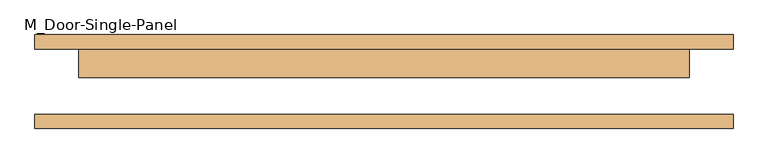
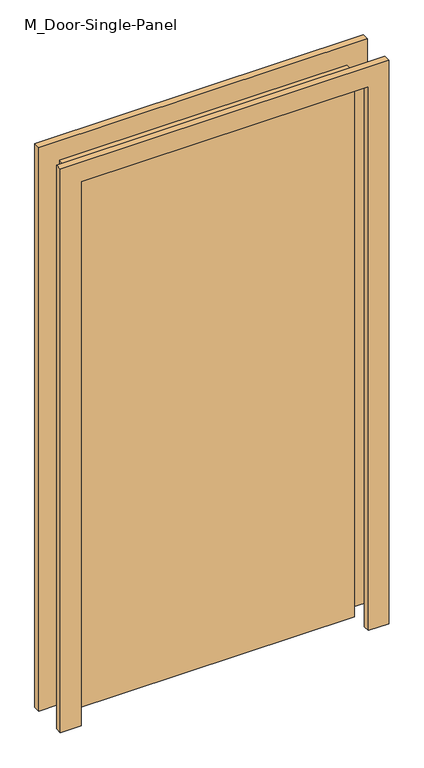
"""IFC4 building model written with IfcOpenShell, lengths in millimetres: door geometry, M_Door-Single-Panel."""

from ifc_helpers import new_model, si_unit, frame, origin, origin_with_axes, place, context, project, spatial, polyline, outline, extrude, source, transform, mapped, element, save


def m_door_single_panel_3722715f(model_context):
    return source(origin(), model_context, "Body", "SweptSolid", [
        extrude(outline(polyline([(533.4, 7.15), (-533.4, 7.15), (-533.4, 57.15), (533.4, 57.15), (533.4, 7.15)])), origin_with_axes(), (0.0, 0.0, 1.0), 2133.6),
        extrude(outline(polyline([(2209.8, 609.6), (2209.8, -609.6), (0.0, -609.6), (0.0, -533.4), (2133.6, -533.4), (2133.6, 533.4), (0.0, 533.4), (0.0, 609.6), (2209.8, 609.6)])), frame((0.0, -82.15, 0.0), z_axis=(0.0, 1.0, 0.0), x_axis=(0.0, 0.0, 1.0)), (0.0, 0.0, 1.0), 25.0),
        extrude(outline(polyline([(2209.8, -609.6), (0.0, -609.6), (0.0, -533.4), (2133.6, -533.4), (2133.6, 533.4), (0.0, 533.4), (0.0, 609.6), (2209.8, 609.6), (2209.8, -609.6)])), frame((0.0, 57.15, 0.0), z_axis=(0.0, 1.0, 0.0), x_axis=(0.0, 0.0, 1.0)), (0.0, 0.0, 1.0), 25.0),
    ])


if __name__ == "__main__":
    model = new_model("IFC4")
    model_context = context("Model", 3, world=origin())
    ifc_project = project(units=[si_unit("LENGTHUNIT", "METRE", prefix="MILLI")], contexts=[model_context])
    site = spatial("IfcSite", under=ifc_project)
    building = spatial("IfcBuilding", under=site)
    placement = place(None, origin())
    m_door_single_panel_shape = m_door_single_panel_3722715f(model_context)
    element("IfcDoor", 1, ObjectType="M_Door-Single-Panel", at=placement, inside=building, context=model_context, shape_type="MappedRepresentation", body=[
        mapped(m_door_single_panel_shape, transform((0.0, 0.0, 0.0), x_axis=(1.0, 0.0, 0.0), y_axis=(0.0, 1.0, 0.0), z_axis=(0.0, 0.0, 1.0))),
    ])
    save(model, "model.ifc")

# Revit data of these elements
# Type "M_Door-Single-Panel"
#   Type Mark = "14"
#   Construction Type Id = "DOOR"
#   Assembly Code = "C1020300"
#   Analytic Construction = "Wooden"
#   Thickness = 0' - 1.9685"
#   Thermal Resistance (R) = 2.5876 (h·ft²·°F)/BTU
#   Swing Angle [instance default] = 90.00°
#   Heat Transfer Coefficient (U) = 0.3865 BTU/(h·ft²·°F)
#   Height = 7' - 0"
#   Trim Projection Ext = 0' - 0.98425"
#   Trim Projection Int = 0' - 0.98425"
#   Trim Width = 0' - 3.14961"
#   Width = 3' - 6"
#   Define Thermal Properties by = 1
#   Panel Material = Wood - Birch - Solid Stained Light Low Gloss
#   Trim Material = Paint - Sienna
#   Visual Light Transmittance = 0
#   Solar Heat Gain Coefficient = 0
#   Function = (empty or 0)
#   Wall Closure = (empty or 0)
# Element 1 (IfcDoor, "M_Door-Single-Panel")
#   Materials on its faces: "Paint - Sienna", "Wood - Birch - Solid Stained Light Low Gloss"
# Materials
#   "Wood - Birch - Solid Stained Light Low Gloss": class "Wood", colour RGB 210 159 95, transparency 0, Cost = 0
#   "Paint - Sienna": colour RGB 118 70 51, transparency 0, Cost = 0
